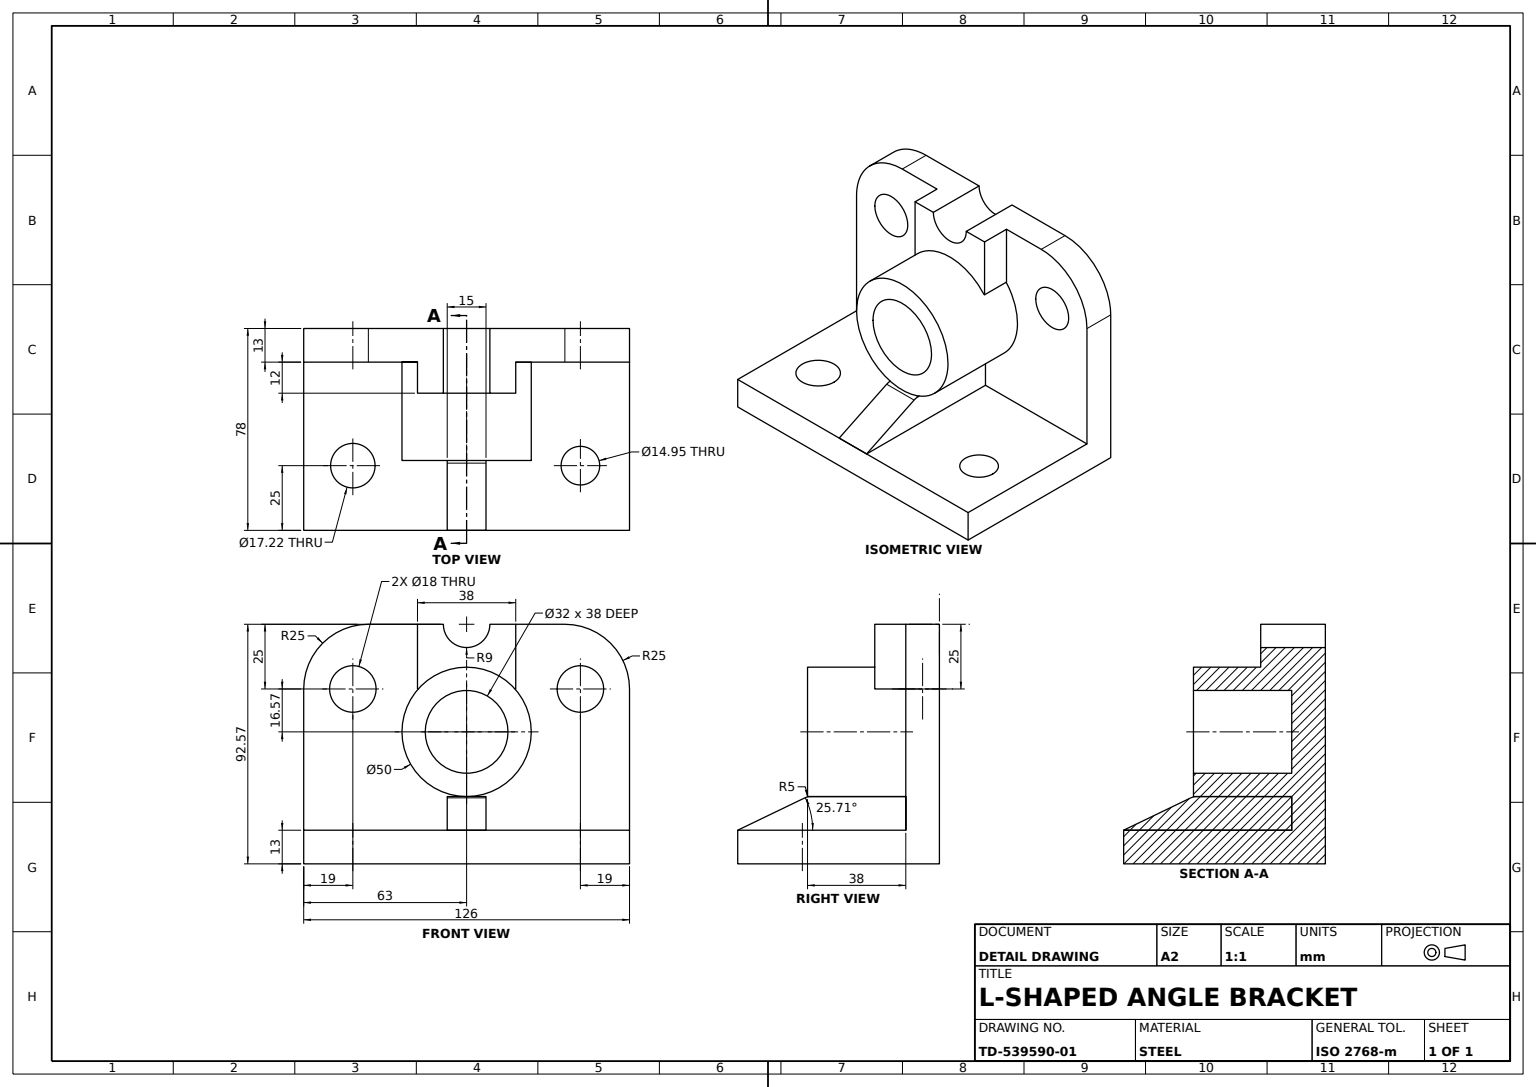
from build123d import *

# Parameters (mm, degrees)
BASE_PLATE_SKETCH_W           = 78
BASE_PLATE_SKETCH_H           = 126
BASE_PLATE_126X78X13_DEPTH    = 13
UPRIGHT_PLATE_SKETCH_W        = 126
UPRIGHT_PLATE_SKETCH_H        = 92.574334666
UPRIGHT_PLATE_DEPTH           = 13
UPRIGHT_CORNER_FILLET_R25_A_R = 25
UPRIGHT_CORNER_FILLET_R25_B_R = 25
UPRIGHT_TOP_BLOCK_DEPTH       = 25
TOP_NOTCH_SKETCH_R            = 9
TOP_NOTCH_18_DEPTH            = 25
UPRIGHT_HOLES_SKETCH_R        = 9
UPRIGHT_HOLES_2X_DEPTH        = 25
BASE_HOLES_SKETCH_R           = 7.472538325
BASE_HOLES_SKETCH_R_2         = 8.609088436
BASE_MOUNTING_HOLES_2X_DEPTH  = 25
HUB_BOSS_SKETCH_R             = 25
HUB_BOSS_DEPTH                = 38
HUB_BORE_SKETCH_R             = 16
HUB_BORE_DEPTH                = 38
GUSSET_RIB_DEPTH              = 7.5
GUSSET_RIB_FILLET_R5_R        = 5


with BuildPart() as part:
    # Base Plate Sketch → Base Plate 126x78x13 (new body)
    with BuildSketch(Plane(origin=(0, 0, 0), x_dir=(1, 0, 0), z_dir=(0, 1, 0))):
        Rectangle(BASE_PLATE_SKETCH_W, BASE_PLATE_SKETCH_H)
    extrude(amount=BASE_PLATE_126X78X13_DEPTH)

    # Upright Plate Sketch → Upright Plate (add)
    with BuildSketch(Plane.ZY.offset(39)):
        with Locations((0, 46.287167333)):
            Rectangle(UPRIGHT_PLATE_SKETCH_W, UPRIGHT_PLATE_SKETCH_H)
    extrude(amount=-UPRIGHT_PLATE_DEPTH)

    # Upright Corner Fillet R25 A
    upright_corner_fillet_r25_a_edges = [part.edges().sort_by_distance(p)[0] for p in [
        (-32.5, 92.574334666, 63),
    ]]
    fillet(upright_corner_fillet_r25_a_edges, radius=UPRIGHT_CORNER_FILLET_R25_A_R)

    # Upright Corner Fillet R25 B
    upright_corner_fillet_r25_b_edges = [part.edges().sort_by_distance(p)[0] for p in [
        (-32.5, 92.574334666, -63),
    ]]
    fillet(upright_corner_fillet_r25_b_edges, radius=UPRIGHT_CORNER_FILLET_R25_B_R)

    # Upright Top Block Sketch → Upright Top Block (add)
    with BuildSketch(Plane.ZY.offset(39)):
        with BuildLine():
            ThreePointArc((9, 92.574334666), (0, 83.574334666), (-9, 92.574334666))
            Line((-9, 92.574334666), (-19, 92.574334666))
            Line((-19, 92.574334666), (-19, 67.574334666))
            Line((-19, 67.574334666), (19, 67.574334666))
            Line((19, 67.574334666), (19, 92.574334666))
            Line((19, 92.574334666), (9, 92.574334666))
        make_face()
    extrude(amount=-UPRIGHT_TOP_BLOCK_DEPTH)

    # Top Notch Sketch → Top Notch Ø18 (cut)
    with BuildSketch(Plane.ZY.offset(39)):
        with Locations((0, 92.574334666)):
            Circle(TOP_NOTCH_SKETCH_R)
    extrude(amount=-TOP_NOTCH_18_DEPTH, mode=Mode.SUBTRACT)

    # Upright Holes Sketch → Upright Holes 2x (cut)
    with BuildSketch(Plane(origin=(-26, 0, 0), x_dir=(0, 0, -1), z_dir=(1, 0, 0))):
        with Locations((-44, 67.574334666)):
            Circle(UPRIGHT_HOLES_SKETCH_R)
        with Locations((44, 67.574334666)):
            Circle(UPRIGHT_HOLES_SKETCH_R)
    extrude(amount=-UPRIGHT_HOLES_2X_DEPTH, mode=Mode.SUBTRACT)

    # Base Holes Sketch → Base Mounting Holes 2x (cut)
    with BuildSketch(Plane(origin=(0, 13, 0), x_dir=(1, 0, 0), z_dir=(0, 1, 0))):
        with Locations(Location((14, 44, 0), (0, 0, 270))):
            Circle(BASE_HOLES_SKETCH_R)
        with Locations(Location((14, -44, 0), (0, 0, 270))):
            Circle(BASE_HOLES_SKETCH_R_2)
    extrude(amount=-BASE_MOUNTING_HOLES_2X_DEPTH, mode=Mode.SUBTRACT)

    # Hub Boss Sketch → Hub Boss (add)
    with BuildSketch(Plane(origin=(-26, 0, 0), x_dir=(0, 0, -1), z_dir=(1, 0, 0))):
        with Locations(Location((0, 51, 0), (0, 0, 138.472963652))):
            Circle(HUB_BOSS_SKETCH_R)
    extrude(amount=HUB_BOSS_DEPTH)

    # Hub Bore Sketch → Hub Bore (cut)
    with BuildSketch(Plane(origin=(12, 0, 0), x_dir=(0, 0, -1), z_dir=(1, 0, 0))):
        with Locations((0, 51)):
            Circle(HUB_BORE_SKETCH_R)
    extrude(amount=-HUB_BORE_DEPTH, mode=Mode.SUBTRACT)


with BuildPart() as body_2:
    # Gusset Rib Sketch → Gusset Rib (new, symmetric)
    with BuildSketch(Plane.XY):
        Polygon((-26, 26), (12, 26), (39, 13), (-26, 13), align=None)
    extrude(amount=GUSSET_RIB_DEPTH, both=True)

    # Gusset Rib Fillet R5
    gusset_rib_fillet_r5_edges = [body_2.edges().sort_by_distance(p)[0] for p in [
        (12, 26, 0),
    ]]
    fillet(gusset_rib_fillet_r5_edges, radius=GUSSET_RIB_FILLET_R5_R)


solid = Compound([part.part, body_2.part])
